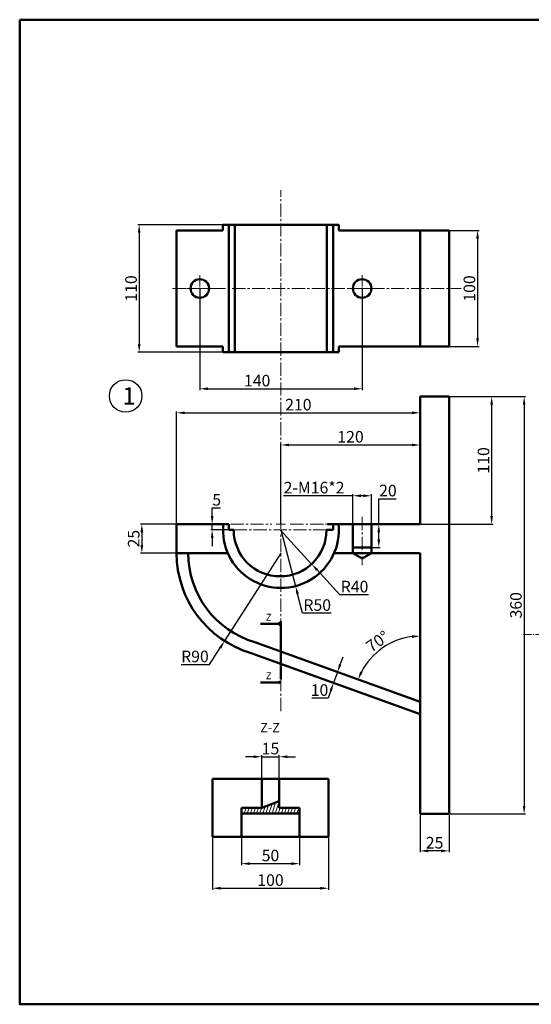
# Model space of a CAD drawing. Units: millimetres. Extents: x -68 to 1086, y -293 to 557.
# Tile 1 of 4: x -68 to 373, y -293 to 557. Entities that reach past the tile are written whole.
import ezdxf

# ---------------------------------------------------------------- set-up
doc = ezdxf.new("R2010")
doc.units = ezdxf.units.MM
doc.header["$LTSCALE"] = 0.6
doc.linetypes.add('CENTER2', pattern=[28.575, 19.05, -3.175, 3.175, -3.175])
for name, color, linetype, lineweight in [('M-CNTR', 1, 'CENTER2', 18), ('M-DIMS', 2, 'Continuous', 25), ('M-HATC', 8, 'Continuous', 18), ('M-OUTL', 7, 'Continuous', 50), ('M-SECT', 6, 'Continuous', 35), ('M-SYMB', 4, 'Continuous', 25), ('M-TEXT', 3, 'Continuous', 25)]:
    doc.layers.add(name, color=color, linetype=linetype, lineweight=lineweight)
doc.styles.get("Standard").update_dxf_attribs({"font": 'arial.ttf'})
doc.dimstyles.new('ISO-25', dxfattribs={"dimtxt": 10, "dimasz": 7, "dimexe": 1.25, "dimexo": 0.625, "dimtad": 1, "dimtoh": 1, "dimtxsty": 'Standard', "dimcen": 2.5, "dimadec": 0, "dimazin": 0, "dimtfac": 1, "dimtmove": 0, "dimatfit": 3, "dimfxl": 1, "dimarcsym": 0})

# ---------------------------------------------------------------- blocks, each defined once
blk = doc.blocks.new('*U1')
at = {"layer": 'M-CNTR', "color": 0, "transparency": 16777216}
for p, q in [((0, 8), (0, 288.21)), ((-43.5, 0), (-8, 0)), ((8, 0), (43.5, 0)), ((0, -161.31), (0, -8))]:
    blk.add_line(p, q, dxfattribs=at)
at = {"layer": 'M-CNTR', "color": 0, "linetype": 'Continuous', "transparency": 16777216}
for p, q in [((-4, 0), (4, 0)), ((0, -4), (0, 4))]:
    blk.add_line(p, q, dxfattribs=at)
blk = doc.blocks.new('*U2')
at = {"layer": 'M-CNTR', "color": 0, "transparency": 16777216}
blk.add_line((-23.5, 0), (225.49, 0), dxfattribs=at)
blk = doc.blocks.new('*U3')
at = {"layer": 'M-CNTR', "color": 0, "transparency": 16777216}
for p, q in [((0, 1.6), (0, 11.5)), ((-11.5, 0), (-1.6, 0)), ((1.6, 0), (11.5, 0)), ((0, -11.5), (0, -1.6))]:
    blk.add_line(p, q, dxfattribs=at)
at = {"layer": 'M-CNTR', "color": 0, "linetype": 'Continuous', "transparency": 16777216}
for p, q in [((-0.8, 0), (0.8, 0)), ((0, -0.8), (0, 0.8))]:
    blk.add_line(p, q, dxfattribs=at)
blk = doc.blocks.new('*U4')
at = {"layer": 'M-CNTR', "color": 0, "transparency": 16777216}
for p, q in [((0, 1.6), (0, 11.5)), ((-11.5, 0), (-1.6, 0)), ((1.6, 0), (11.5, 0)), ((0, -11.5), (0, -1.6))]:
    blk.add_line(p, q, dxfattribs=at)
at = {"layer": 'M-CNTR', "color": 0, "linetype": 'Continuous', "transparency": 16777216}
for p, q in [((-0.8, 0), (0.8, 0)), ((0, -0.8), (0, 0.8))]:
    blk.add_line(p, q, dxfattribs=at)
blk = doc.blocks.new('*D5')
at = {"layer": 'Defpoints', "color": 0, "ltscale": 0.6, "transparency": 16777216}
for p in [(301.93, 231.45), (276.93, 121.45), (338.64, 121.45)]:
    blk.add_point(p, dxfattribs=at)
at = {"layer": 'M-DIMS', "color": 0, "lineweight": -2, "ltscale": 0.6, "transparency": 16777216}
for p, q in [((302.56, 231.45), (339.89, 231.45)), ((338.64, 224.45), (338.64, 128.45)), ((277.56, 121.45), (339.89, 121.45))]:
    blk.add_line(p, q, dxfattribs=at)
at = {"layer": 'M-DIMS', "color": 0, "ltscale": 0.6, "transparency": 16777216}
for points in [[(337.47, 224.45), (339.8, 224.45), (338.64, 231.45)], [(337.47, 128.45), (339.8, 128.45), (338.64, 121.45)]]:
    blk.add_solid(points, dxfattribs=at)
at = {"layer": 'M-DIMS', "color": 0, "ltscale": 0.6, "transparency": 16777216, "insert": (332.91, 176.45), "char_height": 10, "attachment_point": 5, "rotation": 90}
blk.add_mtext('110', dxfattribs=at)
blk = doc.blocks.new('*D6')
at = {"layer": 'Defpoints', "color": 0, "ltscale": 0.6, "transparency": 16777216}
for p in [(276.93, -128.55), (301.93, -128.55), (276.93, -160.38)]:
    blk.add_point(p, dxfattribs=at)
at = {"layer": 'M-DIMS', "color": 0, "lineweight": -2, "ltscale": 0.6, "transparency": 16777216}
for p, q in [((276.93, -129.17), (276.93, -161.63)), ((301.93, -129.17), (301.93, -161.63)), ((294.93, -160.38), (283.93, -160.38))]:
    blk.add_line(p, q, dxfattribs=at)
at = {"layer": 'M-DIMS', "color": 0, "ltscale": 0.6, "transparency": 16777216}
for points in [[(283.93, -159.21), (283.93, -161.55), (276.93, -160.38)], [(294.93, -159.21), (294.93, -161.55), (301.93, -160.38)]]:
    blk.add_solid(points, dxfattribs=at)
at = {"layer": 'M-DIMS', "color": 0, "ltscale": 0.6, "transparency": 16777216, "insert": (289.43, -154.65), "char_height": 10, "attachment_point": 5}
blk.add_mtext('25', dxfattribs=at)
blk = doc.blocks.new('*D7')
at = {"layer": 'Defpoints', "color": 0, "ltscale": 0.6, "transparency": 16777216}
for p in [(301.93, 231.45), (301.93, -128.55), (366.62, -128.55)]:
    blk.add_point(p, dxfattribs=at)
at = {"layer": 'M-DIMS', "color": 0, "lineweight": -2, "ltscale": 0.6, "transparency": 16777216}
for p, q in [((302.56, 231.45), (367.87, 231.45)), ((366.62, 224.45), (366.62, -121.55)), ((302.56, -128.55), (367.87, -128.55))]:
    blk.add_line(p, q, dxfattribs=at)
at = {"layer": 'M-DIMS', "color": 0, "ltscale": 0.6, "transparency": 16777216}
for points in [[(365.46, 224.45), (367.79, 224.45), (366.62, 231.45)], [(365.46, -121.55), (367.79, -121.55), (366.62, -128.55)]]:
    blk.add_solid(points, dxfattribs=at)
at = {"layer": 'M-DIMS', "color": 0, "ltscale": 0.6, "transparency": 16777216, "insert": (360.89, 51.45), "char_height": 10, "attachment_point": 5, "rotation": 90}
blk.add_mtext('360', dxfattribs=at)
blk = doc.blocks.new('*D8')
at = {"layer": 'Defpoints', "color": 0, "ltscale": 0.6, "transparency": 16777216}
for p in [(66.93, 121.45), (36.95, 96.45), (66.93, 96.45)]:
    blk.add_point(p, dxfattribs=at)
at = {"layer": 'M-DIMS', "color": 0, "lineweight": -2, "ltscale": 0.6, "transparency": 16777216}
for p, q in [((66.31, 121.45), (35.7, 121.45)), ((36.95, 114.45), (36.95, 103.45)), ((66.31, 96.45), (35.7, 96.45))]:
    blk.add_line(p, q, dxfattribs=at)
at = {"layer": 'M-DIMS', "color": 0, "ltscale": 0.6, "transparency": 16777216}
for points in [[(35.78, 114.45), (38.12, 114.45), (36.95, 121.45)], [(35.78, 103.45), (38.12, 103.45), (36.95, 96.45)]]:
    blk.add_solid(points, dxfattribs=at)
at = {"layer": 'M-DIMS', "color": 0, "ltscale": 0.6, "transparency": 16777216, "insert": (31.22, 108.95), "char_height": 10, "attachment_point": 5, "rotation": 90}
blk.add_mtext('25', dxfattribs=at)
blk = doc.blocks.new('*D9')
at = {"layer": 'Defpoints', "color": 0, "ltscale": 0.6, "transparency": 16777216}
for p in [(301.93, 374.75), (301.93, 274.75), (326.48, 274.75)]:
    blk.add_point(p, dxfattribs=at)
at = {"layer": 'M-DIMS', "color": 0, "lineweight": -2, "ltscale": 0.6, "transparency": 16777216}
for p, q in [((302.56, 374.75), (327.73, 374.75)), ((326.48, 367.75), (326.48, 281.75)), ((302.56, 274.75), (327.73, 274.75))]:
    blk.add_line(p, q, dxfattribs=at)
at = {"layer": 'M-DIMS', "color": 0, "ltscale": 0.6, "transparency": 16777216}
for points in [[(325.31, 367.75), (327.65, 367.75), (326.48, 374.75)], [(325.31, 281.75), (327.65, 281.75), (326.48, 274.75)]]:
    blk.add_solid(points, dxfattribs=at)
at = {"layer": 'M-DIMS', "color": 0, "ltscale": 0.6, "transparency": 16777216, "insert": (320.75, 324.75), "char_height": 10, "attachment_point": 5, "rotation": 90}
blk.add_mtext('100', dxfattribs=at)
blk = doc.blocks.new('*D10')
at = {"layer": 'Defpoints', "color": 0, "ltscale": 0.6, "transparency": 16777216}
for p in [(180.89, 379.75), (34.66, 269.75), (180.89, 269.75)]:
    blk.add_point(p, dxfattribs=at)
at = {"layer": 'M-DIMS', "color": 0, "lineweight": -2, "ltscale": 0.6, "transparency": 16777216}
for p, q in [((180.26, 379.75), (33.41, 379.75)), ((34.66, 372.75), (34.66, 276.75)), ((180.26, 269.75), (33.41, 269.75))]:
    blk.add_line(p, q, dxfattribs=at)
at = {"layer": 'M-DIMS', "color": 0, "ltscale": 0.6, "transparency": 16777216}
for points in [[(33.49, 372.75), (35.82, 372.75), (34.66, 379.75)], [(33.49, 276.75), (35.82, 276.75), (34.66, 269.75)]]:
    blk.add_solid(points, dxfattribs=at)
at = {"layer": 'M-DIMS', "color": 0, "ltscale": 0.6, "transparency": 16777216, "insert": (28.93, 324.75), "char_height": 10, "attachment_point": 5, "rotation": 90}
blk.add_mtext('110', dxfattribs=at)
blk = doc.blocks.new('*D11')
at = {"layer": 'Defpoints', "color": 0, "ltscale": 0.6, "transparency": 16777216}
for p in [(86.93, 324.75), (226.93, 324.75), (226.93, 238.25)]:
    blk.add_point(p, dxfattribs=at)
at = {"layer": 'M-DIMS', "color": 0, "lineweight": -2, "ltscale": 0.6, "transparency": 16777216}
for p, q in [((86.93, 324.13), (86.93, 237)), ((226.93, 324.13), (226.93, 237)), ((93.93, 238.25), (219.93, 238.25))]:
    blk.add_line(p, q, dxfattribs=at)
at = {"layer": 'M-DIMS', "color": 0, "ltscale": 0.6, "transparency": 16777216}
for points in [[(93.93, 239.41), (93.93, 237.08), (86.93, 238.25)], [(219.93, 239.41), (219.93, 237.08), (226.93, 238.25)]]:
    blk.add_solid(points, dxfattribs=at)
at = {"layer": 'M-DIMS', "color": 0, "ltscale": 0.6, "transparency": 16777216, "insert": (136.43, 243.98), "char_height": 10, "attachment_point": 5}
blk.add_mtext('140', dxfattribs=at)
blk = doc.blocks.new('*D12')
at = {"layer": 'Defpoints', "color": 0, "ltscale": 0.6, "transparency": 16777216}
for p in [(156.93, 96.45), (108.36, 20.68)]:
    blk.add_point(p, dxfattribs=at)
at = {"layer": 'M-DIMS', "color": 0, "lineweight": -2, "ltscale": 0.6, "transparency": 16777216}
for p, q in [((156.93, 96.45), (108.36, 20.68)), ((95.3, 0.3), (104.58, 14.79)), ((70.81, 0.3), (95.3, 0.3))]:
    blk.add_line(p, q, dxfattribs=at)
at = {"layer": 'M-DIMS', "color": 0, "ltscale": 0.6, "transparency": 16777216}
blk.add_solid([(103.6, 15.42), (105.57, 14.16), (108.36, 20.68)], dxfattribs=at)
at = {"layer": 'M-DIMS', "color": 0, "ltscale": 0.6, "transparency": 16777216, "insert": (82.74, 6.03), "char_height": 10, "attachment_point": 5}
blk.add_mtext('R90', dxfattribs=at)
blk = doc.blocks.new('*D13')
at = {"layer": 'Defpoints', "color": 0, "ltscale": 0.6, "transparency": 16777216}
for p in [(276.93, 217.49), (66.93, 121.45), (276.93, 121.45)]:
    blk.add_point(p, dxfattribs=at)
at = {"layer": 'M-DIMS', "color": 0, "lineweight": -2, "ltscale": 0.6, "transparency": 16777216}
for p, q in [((66.93, 122.08), (66.93, 218.74)), ((73.93, 217.49), (269.93, 217.49)), ((276.93, 122.08), (276.93, 218.74))]:
    blk.add_line(p, q, dxfattribs=at)
at = {"layer": 'M-DIMS', "color": 0, "ltscale": 0.6, "transparency": 16777216}
for points in [[(73.93, 218.65), (73.93, 216.32), (66.93, 217.49)], [(269.93, 218.65), (269.93, 216.32), (276.93, 217.49)]]:
    blk.add_solid(points, dxfattribs=at)
at = {"layer": 'M-DIMS', "color": 0, "ltscale": 0.6, "transparency": 16777216, "insert": (171.93, 223.22), "char_height": 10, "attachment_point": 5}
blk.add_mtext('210', dxfattribs=at)
blk = doc.blocks.new('*D14')
at = {"layer": 'Defpoints', "color": 0, "ltscale": 0.6, "transparency": 16777216}
for p in [(276.93, 189.78), (156.93, 121.45), (276.93, 121.45)]:
    blk.add_point(p, dxfattribs=at)
at = {"layer": 'M-DIMS', "color": 0, "lineweight": -2, "ltscale": 0.6, "transparency": 16777216}
for p, q in [((156.93, 122.08), (156.93, 191.03)), ((163.93, 189.78), (269.93, 189.78)), ((276.93, 122.08), (276.93, 191.03))]:
    blk.add_line(p, q, dxfattribs=at)
at = {"layer": 'M-DIMS', "color": 0, "ltscale": 0.6, "transparency": 16777216}
for points in [[(163.93, 190.94), (163.93, 188.61), (156.93, 189.78)], [(269.93, 190.94), (269.93, 188.61), (276.93, 189.78)]]:
    blk.add_solid(points, dxfattribs=at)
at = {"layer": 'M-DIMS', "color": 0, "ltscale": 0.6, "transparency": 16777216, "insert": (216.93, 195.51), "char_height": 10, "attachment_point": 5}
blk.add_mtext('120', dxfattribs=at)
blk = doc.blocks.new('*D15')
at = {"layer": 'Defpoints', "color": 0, "ltscale": 0.6, "transparency": 16777216}
for p in [(234.93, 121.45), (241.32, 121.45), (234.93, 101.45)]:
    blk.add_point(p, dxfattribs=at)
at = {"layer": 'M-DIMS', "color": 0, "lineweight": -2, "ltscale": 0.6, "transparency": 16777216}
for p, q in [((241.32, 121.45), (241.32, 143.38)), ((241.32, 143.38), (256.41, 143.38)), ((235.56, 121.45), (242.57, 121.45)), ((241.32, 108.45), (241.32, 114.45)), ((235.56, 101.45), (242.57, 101.45))]:
    blk.add_line(p, q, dxfattribs=at)
at = {"layer": 'M-DIMS', "color": 0, "ltscale": 0.6, "transparency": 16777216}
for points in [[(240.15, 114.45), (242.49, 114.45), (241.32, 121.45)], [(240.15, 108.45), (242.49, 108.45), (241.32, 101.45)]]:
    blk.add_solid(points, dxfattribs=at)
at = {"layer": 'M-DIMS', "color": 0, "ltscale": 0.6, "transparency": 16777216, "insert": (249.17, 149.11), "char_height": 10, "attachment_point": 5}
blk.add_mtext('20', dxfattribs=at)
blk = doc.blocks.new('*D16')
at = {"layer": 'Defpoints', "color": 0, "ltscale": 0.6, "transparency": 16777216}
for p in [(218.93, 145.93), (218.93, 121.45), (234.93, 121.45)]:
    blk.add_point(p, dxfattribs=at)
at = {"layer": 'M-DIMS', "color": 0, "lineweight": -2, "ltscale": 0.6, "transparency": 16777216}
for p, q in [((218.93, 145.93), (159.03, 145.93)), ((218.93, 122.08), (218.93, 147.18)), ((227.93, 145.93), (225.93, 145.93)), ((234.93, 122.08), (234.93, 147.18))]:
    blk.add_line(p, q, dxfattribs=at)
at = {"layer": 'M-DIMS', "color": 0, "ltscale": 0.6, "transparency": 16777216}
for points in [[(225.93, 147.1), (225.93, 144.76), (218.93, 145.93)], [(227.93, 147.1), (227.93, 144.76), (234.93, 145.93)]]:
    blk.add_solid(points, dxfattribs=at)
at = {"layer": 'M-DIMS', "color": 0, "ltscale": 0.6, "transparency": 16777216, "insert": (185.48, 151.66), "char_height": 10, "attachment_point": 5}
blk.add_mtext('2-M16*2', dxfattribs=at)
blk = doc.blocks.new('*D17')
at = {"layer": 'Defpoints', "color": 0, "ltscale": 0.6, "transparency": 16777216}
for p in [(97.58, 121.45), (111.93, 121.45), (111.93, 116.45)]:
    blk.add_point(p, dxfattribs=at)
at = {"layer": 'M-DIMS', "color": 0, "lineweight": -2, "ltscale": 0.6, "transparency": 16777216}
for p, q in [((97.58, 128.45), (97.58, 135.45)), ((97.58, 135.45), (104.84, 135.45)), ((111.31, 121.45), (96.33, 121.45)), ((97.58, 116.45), (97.58, 121.45)), ((111.31, 116.45), (96.33, 116.45)), ((97.58, 109.45), (97.58, 102.45))]:
    blk.add_line(p, q, dxfattribs=at)
at = {"layer": 'M-DIMS', "color": 0, "ltscale": 0.6, "transparency": 16777216}
for points in [[(96.42, 128.45), (98.75, 128.45), (97.58, 121.45)], [(96.42, 109.45), (98.75, 109.45), (97.58, 116.45)]]:
    blk.add_solid(points, dxfattribs=at)
at = {"layer": 'M-DIMS', "color": 0, "ltscale": 0.6, "transparency": 16777216, "insert": (101.52, 141.16), "char_height": 10, "attachment_point": 5}
blk.add_mtext('5', dxfattribs=at)
blk = doc.blocks.new('*D18')
at = {"layer": 'Defpoints', "color": 0, "ltscale": 0.6, "transparency": 16777216}
for p in [(205.67, -6.13), (202.26, -15.53), (202.26, -15.53)]:
    blk.add_point(p, dxfattribs=at)
at = {"layer": 'M-DIMS', "color": 0, "lineweight": -2, "ltscale": 0.6, "transparency": 16777216}
for p, q in [((208.06, 0.45), (210.44, 7.03)), ((205.67, -6.13), (202.26, -15.53)), ((205.08, -5.92), (204.5, -5.7)), ((201.68, -15.32), (201.09, -15.1)), ((199.88, -22.11), (197.5, -28.69)), ((197.5, -28.69), (183.52, -28.69))]:
    blk.add_line(p, q, dxfattribs=at)
at = {"layer": 'M-DIMS', "color": 0, "ltscale": 0.6, "transparency": 16777216}
for points in [[(206.96, 0.85), (209.15, 0.06), (205.67, -6.13)], [(198.78, -21.71), (200.98, -22.51), (202.26, -15.53)]]:
    blk.add_solid(points, dxfattribs=at)
at = {"layer": 'M-DIMS', "color": 0, "ltscale": 0.6, "transparency": 16777216, "insert": (190.2, -22.96), "char_height": 10, "attachment_point": 5}
blk.add_mtext('10', dxfattribs=at)
blk = doc.blocks.new('*D19')
at = {"layer": 'Defpoints', "color": 0, "ltscale": 0.6, "transparency": 16777216}
for p in [(276.93, 96.45), (134.41, 19.69), (254.4, 20.23), (276.93, -31.95), (276.93, -128.55)]:
    blk.add_point(p, dxfattribs=at)
at = {"layer": 'M-DIMS', "color": 0, "lineweight": -2, "ltscale": 0.6, "transparency": 16777216}
blk.add_arc((276.93, -31.95), 56.84, 97.06102, 153.02444, dxfattribs=at)
at = {"layer": 'M-DIMS', "color": 0, "ltscale": 0.6, "transparency": 16777216}
for points in [[(269.87, 25.62), (270.02, 23.3), (276.93, 24.89)], [(227.35, -6.63), (225.21, -5.7), (223.5, -12.59)]]:
    blk.add_solid(points, dxfattribs=at)
at = {"layer": 'M-DIMS', "color": 0, "ltscale": 0.6, "transparency": 16777216, "insert": (241.01, 19.28), "char_height": 10, "attachment_point": 5, "rotation": 35.04273}
blk.add_mtext('70°', dxfattribs=at)
blk = doc.blocks.new('*D20')
at = {"layer": 'Defpoints', "color": 0, "ltscale": 0.6, "transparency": 16777216}
for p in [(156.18, 116.45), (183.33, 87.07)]:
    blk.add_point(p, dxfattribs=at)
at = {"layer": 'M-DIMS', "color": 0, "lineweight": -2, "ltscale": 0.6, "transparency": 16777216}
for p, q in [((156.18, 116.45), (183.33, 87.07)), ((207.84, 60.54), (188.08, 81.93)), ((232.33, 60.54), (207.84, 60.54))]:
    blk.add_line(p, q, dxfattribs=at)
at = {"layer": 'M-DIMS', "color": 0, "ltscale": 0.6, "transparency": 16777216}
blk.add_solid([(188.94, 82.72), (187.22, 81.14), (183.33, 87.07)], dxfattribs=at)
at = {"layer": 'M-DIMS', "color": 0, "ltscale": 0.6, "transparency": 16777216, "insert": (220.4, 66.27), "char_height": 10, "attachment_point": 5}
blk.add_mtext('R40', dxfattribs=at)
blk = doc.blocks.new('*D21')
at = {"layer": 'Defpoints', "color": 0, "ltscale": 0.6, "transparency": 16777216}
for p in [(156.93, 116.45), (169.54, 68.07)]:
    blk.add_point(p, dxfattribs=at)
at = {"layer": 'M-DIMS', "color": 0, "lineweight": -2, "ltscale": 0.6, "transparency": 16777216}
for p, q in [((156.93, 116.45), (169.54, 68.07)), ((175.65, 44.64), (171.31, 61.3)), ((200.14, 44.64), (175.65, 44.64))]:
    blk.add_line(p, q, dxfattribs=at)
at = {"layer": 'M-DIMS', "color": 0, "ltscale": 0.6, "transparency": 16777216}
blk.add_solid([(172.44, 61.59), (170.18, 61), (169.54, 68.07)], dxfattribs=at)
at = {"layer": 'M-DIMS', "color": 0, "ltscale": 0.6, "transparency": 16777216, "insert": (188.21, 50.37), "char_height": 10, "attachment_point": 5}
blk.add_mtext('R50', dxfattribs=at)
blk = doc.blocks.new('*D68')
at = {"layer": 'Defpoints', "color": 0, "ltscale": 0.6, "transparency": 16777216}
for p in [(122.91, -148.12), (172.91, -148.12), (172.91, -171.36)]:
    blk.add_point(p, dxfattribs=at)
at = {"layer": 'M-DIMS', "color": 0, "lineweight": -2, "ltscale": 0.6, "transparency": 16777216}
for p, q in [((122.91, -148.75), (122.91, -172.61)), ((172.91, -148.75), (172.91, -172.61)), ((129.91, -171.36), (165.91, -171.36))]:
    blk.add_line(p, q, dxfattribs=at)
at = {"layer": 'M-DIMS', "color": 0, "ltscale": 0.6, "transparency": 16777216}
for points in [[(129.91, -170.19), (129.91, -172.53), (122.91, -171.36)], [(165.91, -170.19), (165.91, -172.53), (172.91, -171.36)]]:
    blk.add_solid(points, dxfattribs=at)
at = {"layer": 'M-DIMS', "color": 0, "ltscale": 0.6, "transparency": 16777216, "insert": (147.91, -165.63), "char_height": 10, "attachment_point": 5}
blk.add_mtext('50', dxfattribs=at)
blk = doc.blocks.new('*D69')
at = {"layer": 'Defpoints', "color": 0, "ltscale": 0.6, "transparency": 16777216}
for p in [(97.91, -148.12), (197.91, -148.12), (197.91, -192.61)]:
    blk.add_point(p, dxfattribs=at)
at = {"layer": 'M-DIMS', "color": 0, "lineweight": -2, "ltscale": 0.6, "transparency": 16777216}
for p, q in [((97.91, -148.75), (97.91, -193.86)), ((197.91, -148.75), (197.91, -193.86)), ((104.91, -192.61), (190.91, -192.61))]:
    blk.add_line(p, q, dxfattribs=at)
at = {"layer": 'M-DIMS', "color": 0, "ltscale": 0.6, "transparency": 16777216}
for points in [[(104.91, -191.44), (104.91, -193.77), (97.91, -192.61)], [(190.91, -191.44), (190.91, -193.77), (197.91, -192.61)]]:
    blk.add_solid(points, dxfattribs=at)
at = {"layer": 'M-DIMS', "color": 0, "ltscale": 0.6, "transparency": 16777216, "insert": (147.91, -186.88), "char_height": 10, "attachment_point": 5}
blk.add_mtext('100', dxfattribs=at)
blk = doc.blocks.new('*D70')
at = {"layer": 'Defpoints', "color": 0, "ltscale": 0.6, "transparency": 16777216}
for p in [(155.41, -79.16), (140.41, -98.12), (155.41, -98.12)]:
    blk.add_point(p, dxfattribs=at)
at = {"layer": 'M-DIMS', "color": 0, "lineweight": -2, "ltscale": 0.6, "transparency": 16777216}
for p, q in [((133.41, -79.16), (126.41, -79.16)), ((140.41, -97.5), (140.41, -77.91)), ((140.41, -79.16), (155.41, -79.16)), ((155.41, -97.5), (155.41, -77.91)), ((162.41, -79.16), (169.41, -79.16))]:
    blk.add_line(p, q, dxfattribs=at)
at = {"layer": 'M-DIMS', "color": 0, "ltscale": 0.6, "transparency": 16777216}
for points in [[(133.41, -77.99), (133.41, -80.33), (140.41, -79.16)], [(162.41, -77.99), (162.41, -80.33), (155.41, -79.16)]]:
    blk.add_solid(points, dxfattribs=at)
at = {"layer": 'M-DIMS', "color": 0, "ltscale": 0.6, "transparency": 16777216, "insert": (147.91, -73.43), "char_height": 10, "attachment_point": 5}
blk.add_mtext('15', dxfattribs=at)
blk = doc.blocks.new('SECT-ARROW')
at = {"ltscale": 0.6}
for p, q in [((1.92, 1.11), (0, 2.22)), ((0, 2.22), (0, 0)), ((1.92, 1.11), (0, 0))]:
    blk.add_line(p, q, dxfattribs=at)

msp = doc.modelspace()

# ---------------------------------------------------------------- hatches: boundary and pattern name
at = {"layer": 'M-HATC', "ltscale": 0.6}
h = msp.add_hatch(dxfattribs=at)
h.set_pattern_fill('ANSI31', color=256, scale=0.8, angle=27)
h.set_pattern_definition([(72, (35.2612, 47.1151), (-2.415684, 0.784903), [])])
h.paths.add_polyline_path([(140.405, -123.12), (122.905, -123.12), (122.905, -128.12), (172.905, -128.12), (172.905, -123.12), (155.405, -123.12), (155.405, -117.631)])

# ---------------------------------------------------------------- linework, layer by layer
at = {"layer": 'M-CNTR'}
for p, q in [((226.933, 127.738), (226.933, 86.121)), ((196.183, 116.453), (111.933, 116.453))]:
    msp.add_line(p, q, dxfattribs=at)
at = {"layer": 'M-CNTR', "ltscale": 0.6}
msp.add_line((366.081, 26.275), (668.128, 26.275), dxfattribs=at)
at = {"layer": 'M-OUTL', "ltscale": 0.6}
for p, q in [((66.933, 274.754), (66.933, 374.754)), ((66.933, 374.754), (106.933, 374.754)), ((106.933, 379.754), (206.933, 379.754)), ((106.933, 379.754), (106.933, 374.754)), ((111.933, 379.754), (111.933, 269.754)), ((117.247, 379.754), (117.247, 269.754)), ((196.62, 379.754), (196.62, 269.754)), ((201.933, 379.754), (201.933, 269.754)), ((206.933, 379.754), (206.933, 374.754)), ((206.933, 374.754), (276.933, 374.754)), ((301.933, 374.754), (276.933, 374.754)), ((276.933, 374.754), (276.933, 274.754)), ((301.933, 274.754), (301.933, 374.754)), ((66.933, 274.754), (106.933, 274.754)), ((106.933, 269.754), (106.933, 274.754)), ((206.933, 269.754), (206.933, 274.754)), ((206.933, 274.754), (276.933, 274.754)), ((276.933, 274.754), (301.933, 274.754)), ((106.933, 269.754), (206.933, 269.754)), ((111.933, 116.453), (116.183, 116.453)), ((196.183, 116.453), (200.433, 116.453)), ((218.933, 96.453), (226.933, 91.834)), ((234.933, 96.453), (226.933, 91.834)), ((139.229, 35.385), (155.014, 35.385)), ((156.933, 37.882), (156.933, -12.371)), ((139.229, -15.009), (155.014, -15.009)), ((97.905, -148.12), (97.905, -98.12)), ((97.905, -98.12), (197.905, -98.12)), ((140.405, -123.12), (140.405, -98.12)), ((155.405, -123.12), (155.405, -98.12)), ((197.905, -98.12), (197.905, -148.12)), ((140.405, -123.12), (155.405, -117.631)), ((122.905, -123.12), (122.905, -148.12)), ((140.405, -123.12), (122.905, -123.12)), ((172.905, -123.12), (155.405, -123.12)), ((172.905, -123.12), (172.905, -148.12)), ((172.905, -128.12), (122.905, -128.12)), ((197.905, -148.12), (97.905, -148.12))]:
    msp.add_line(p, q, dxfattribs=at)
at = {"layer": 'M-OUTL'}
for p, q in [((276.933, 121.453), (276.933, 231.453)), ((276.933, 231.453), (301.933, 231.453)), ((301.933, 231.453), (301.933, -128.547)), ((111.933, 121.453), (66.933, 121.453)), ((66.933, 121.453), (66.933, 96.453)), ((111.933, 121.453), (111.933, 116.453)), ((196.933, 121.453), (276.933, 121.453)), ((196.933, 121.453), (201.933, 121.453)), ((201.933, 121.453), (201.933, 116.453)), ((218.933, 121.453), (218.933, 96.453)), ((234.933, 121.453), (234.933, 96.453)), ((196.62, 116.453), (201.933, 116.453)), ((66.933, 96.453), (111.108, 96.453)), ((202.759, 96.453), (276.933, 96.453)), ((218.933, 101.453), (234.933, 101.453)), ((276.933, 96.453), (276.933, -128.547)), ((301.933, -128.547), (276.933, -128.547))]:
    msp.add_line(p, q, dxfattribs=at)
at = {"layer": 'M-OUTL', "ltscale": 0.6}
msp.add_lwpolyline([(-68.392, 556.589), (1085.677, 556.589), (1085.677, -292.72), (-68.392, -292.72)], close=True, dxfattribs=at)
at = {"layer": 'M-OUTL'}
for points in [[(66.933, 96.453, 0.331893), (131.286, 10.184), (276.933, -42.581)], [(76.933, 96.453, 0.33288), (134.408, 19.689), (276.933, -31.945)]]:
    msp.add_lwpolyline(points, format="xyb", dxfattribs=at)
at = {"layer": 'M-OUTL', "ltscale": 0.6}
for centre in [(86.933, 324.754), (226.933, 324.754)]:
    msp.add_circle(centre, 8, dxfattribs=at)
for centre, radius, start, end in [((156.933, 116.453), 50, 174.26083, 5.73917), ((156.183, 116.453), 40, 180, 0)]:
    msp.add_arc(centre, radius, start, end, dxfattribs=at)
at = {"layer": 'M-SYMB', "ltscale": 0.6}
msp.add_circle((22.997, 232.017), 14.053, dxfattribs=at)

# ---------------------------------------------------------------- block references
at = {"layer": 'M-CNTR'}
for name, p in [('*U1', (156.933, 121.453)), ('*U4', (86.933, 324.754)), ('*U3', (226.933, 324.754)), ('*U2', (86.933, 324.754))]:
    msp.add_blockref(name, p, dxfattribs=at)
at = {"layer": 'M-SECT'}
for p in [(155.014, 34.276), (155.014, -16.117)]:
    msp.add_blockref('SECT-ARROW', p, dxfattribs=at)

# ---------------------------------------------------------------- texts
at = {"layer": 'M-TEXT', "ltscale": 0.6, "attachment_point": 1}
for s, width, insert, char_height in [('1', 27.55708, (20.234, 239.548), 15), ('\\pxqc;Z', 10.13963, (141.301, 44.117), 6), ('\\pxqc;Z', 10.13963, (141.301, -6.276), 6), ('Z-Z', 23.26032, (139.079, -49.992), 8)]:
    msp.add_mtext_dynamic_manual_height_columns(s, width=width, gutter_width=12.5, heights=[0], dxfattribs=dict(at, insert=insert, char_height=char_height))

# ---------------------------------------------------------------- dimensions: what is measured, and where the dimension line sits
at = {"layer": 'M-DIMS', "ltscale": 0.6}
for base, p1, p2, picture, middle in [((34.657, 269.754), (180.886, 379.754), (180.886, 269.754), '*D10', (28.926, 324.754)), ((326.48, 274.754), (301.933, 374.754), (301.933, 274.754), '*D9', (320.749, 324.754)), ((338.636, 121.453), (301.933, 231.453), (276.933, 121.453), '*D5', (332.905, 176.453)), ((366.622, -128.547), (301.933, 231.453), (301.933, -128.547), '*D7', (360.888, 51.453)), ((97.584, 121.453), (111.933, 116.453), (111.933, 121.453), '*D17', (101.524, 141.163)), ((36.95, 96.453), (66.933, 121.453), (66.933, 96.453), '*D8', (31.219, 108.953))]:
    dim = msp.add_linear_dim(base=base, p1=p1, p2=p2, angle=90, dimstyle='ISO-25', override={"dimclrd": 0, "dimclre": 0, "dimclrt": 0}, dxfattribs=at)
    dim.commit()
    dim.dimension.update_dxf_attribs({"geometry": picture, "text_midpoint": middle})
for base, p1, p2, override, picture, middle in [((226.933, 238.247), (86.933, 324.754), (226.933, 324.754), {"dimclrd": 0, "dimclre": 0, "dimclrt": 0, "dimtmove": 2}, '*D11', (136.425, 243.978)), ((276.933, -160.381), (301.933, -128.547), (276.933, -128.547), {"dimclrd": 0, "dimclre": 0, "dimclrt": 0}, '*D6', (289.433, -160.381))]:
    dim = msp.add_linear_dim(base=base, p1=p1, p2=p2, dimstyle='ISO-25', override=override, dxfattribs=at)
    dim.commit()
    dim.dimension.update_dxf_attribs({"geometry": picture, "text_midpoint": middle, "dimtype": 160})
for base, p1, p2, picture, middle in [((276.933, 217.488), (66.933, 121.453), (276.933, 121.453), '*D13', (171.933, 223.219)), ((276.933, 189.775), (156.933, 121.453), (276.933, 121.453), '*D14', (216.933, 195.506)), ((155.405, -79.16), (140.405, -98.12), (155.405, -98.12), '*D70', (147.905, -73.429)), ((197.905, -192.608), (97.905, -148.12), (197.905, -148.12), '*D69', (147.905, -186.877)), ((172.905, -171.361), (122.905, -148.12), (172.905, -148.12), '*D68', (147.905, -165.63))]:
    dim = msp.add_linear_dim(base=base, p1=p1, p2=p2, dimstyle='ISO-25', override={"dimclrd": 0, "dimclre": 0, "dimclrt": 0}, dxfattribs=at)
    dim.commit()
    dim.dimension.update_dxf_attribs({"geometry": picture, "text_midpoint": middle})
dim = msp.add_linear_dim(base=(218.933, 145.93), p1=(234.933, 121.453), p2=(218.933, 121.453), text='2-M<>*2', dimstyle='ISO-25', override={"dimclrd": 0, "dimclre": 0, "dimclrt": 0}, dxfattribs=at)
dim.commit()
dim.dimension.update_dxf_attribs({"geometry": '*D16', "text_midpoint": (185.48, 145.93), "dimtype": 160})
dim = msp.add_linear_dim(base=(241.319, 121.453), p1=(234.933, 101.453), p2=(234.933, 121.453), angle=90, dimstyle='ISO-25', override={"dimclrd": 0, "dimclre": 0, "dimclrt": 0}, dxfattribs=at)
dim.commit()
dim.dimension.update_dxf_attribs({"geometry": '*D15', "text_midpoint": (249.175, 143.377), "dimtype": 160})
dim = msp.add_radius_dim(center=(156.183, 116.453), mpoint=(183.328, 87.073), dimstyle='ISO-25', override={"dimclrd": 0, "dimclre": 0, "dimclrt": 0}, dxfattribs=at)
dim.commit()
dim.dimension.update_dxf_attribs({"geometry": '*D20', "text_midpoint": (220.396, 60.542), "dimtype": 164})
for center, mpoint, picture, middle in [((156.933, 116.453), (169.544, 68.069), '*D21', (188.206, 50.371)), ((156.933, 96.453), (108.362, 20.685), '*D12', (82.74, 6.033))]:
    dim = msp.add_radius_dim(center=center, mpoint=mpoint, dimstyle='ISO-25', override={"dimclrd": 0, "dimclre": 0, "dimclrt": 0}, dxfattribs=at)
    dim.commit()
    dim.dimension.update_dxf_attribs({"geometry": picture, "text_midpoint": middle})
dim = msp.add_angular_dim_2l(base=(254.396, 20.232), line1=((276.933, 96.453), (276.933, -128.547)), line2=((134.408, 19.689), (276.933, -31.945)), dimstyle='ISO-25', override={"dimclrd": 0, "dimclre": 0, "dimclrt": 0}, dxfattribs=at)
dim.commit()
dim.dimension.update_dxf_attribs({"geometry": '*D19', "text_midpoint": (241.008, 19.28)})
dim = msp.add_aligned_dim(p1=(205.671, -6.128), p2=(202.265, -15.53), distance=0, dimstyle='ISO-25', override={"dimclrd": 0, "dimclre": 0, "dimclrt": 0}, dxfattribs=at)
dim.commit()
dim.dimension.update_dxf_attribs({"geometry": '*D18', "text_midpoint": (190.196, -22.962)})

doc.saveas('drawing.dxf')
